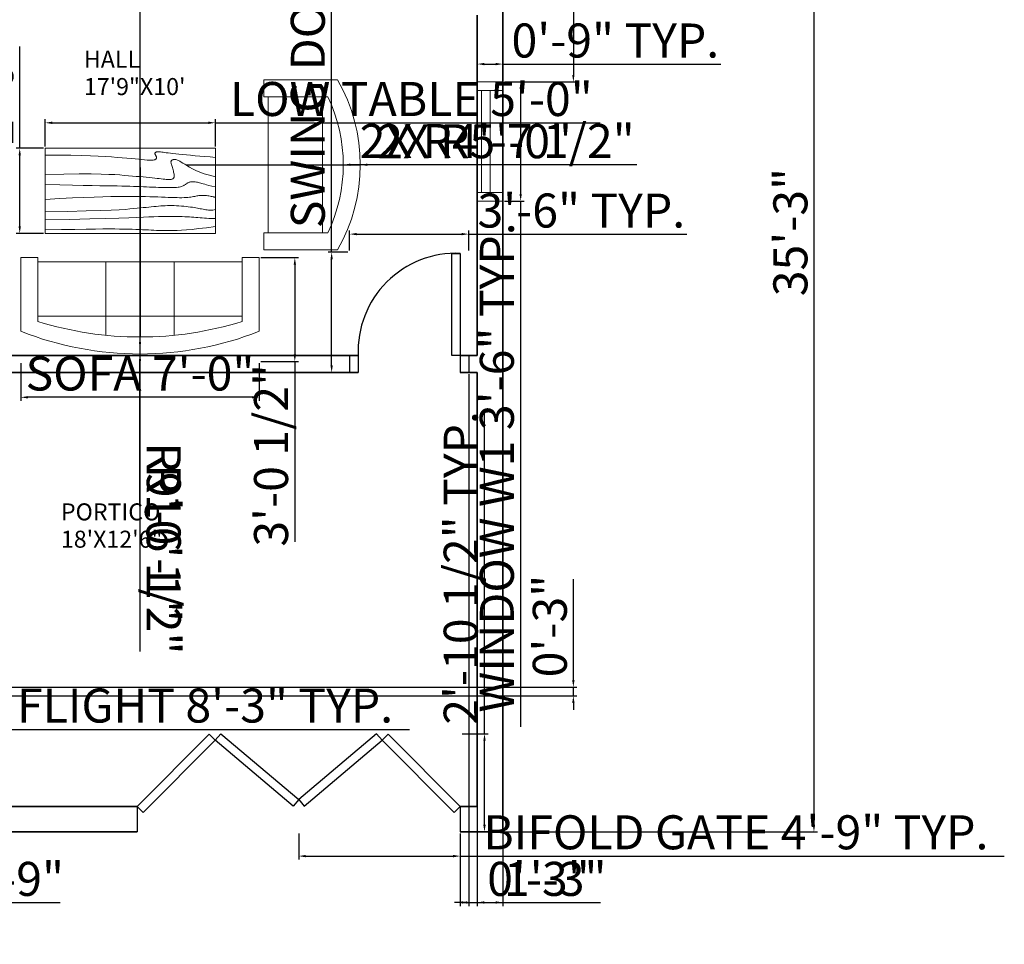
# Model space of a CAD drawing. Units: inches. Extents: x 2330 to 2931, y 514 to 1098.
# Tile 3 of 4: x 2583 to 2931, y 559 to 885. Entities that reach past the tile are written whole.
import ezdxf

# ---------------------------------------------------------------- set-up
doc = ezdxf.new("R2010")
doc.units = ezdxf.units.IN
for name, color, linetype, lineweight in [('A-ANNO-DIMS', 2, 'Continuous', 18), ('A-AREA-IDEN', 7, 'Continuous', 18), ('A-DOOR', 3, 'Continuous', 25), ('A-FURN', 8, 'Continuous', 18), ('A-GLAZ', 4, 'Continuous', 18), ('A-WALL', 7, 'Continuous', 35)]:
    doc.layers.add(name, color=color, linetype=linetype, lineweight=lineweight)
doc.styles.get("Standard").update_dxf_attribs({"font": 'arial.ttf'})
doc.dimstyles.new('ISO-25', dxfattribs={"dimtxt": 12, "dimasz": 2.5, "dimexe": 1.25, "dimexo": 0.625, "dimtad": 1, "dimdec": 1, "dimlunit": 3, "dimtxsty": 'Standard', "dimcen": 2.5, "dimadec": 0, "dimazin": 0, "dimtfac": 1, "dimtdec": 1, "dimtmove": 0, "dimatfit": 3, "dimfxl": 1, "dimarcsym": 0})

# ---------------------------------------------------------------- blocks, each defined once
blk = doc.blocks.new('*D2')
at = {"layer": 'A-ANNO-DIMS', "color": 0, "lineweight": -2, "transparency": 16777216}
for p, q in [((2754.43, 1021.47), (2864.79, 1021.47)), ((2863.54, 1018.97), (2863.54, 600.97)), ((2754.43, 598.47), (2864.79, 598.47))]:
    blk.add_line(p, q, dxfattribs=at)
at = {"layer": 'A-ANNO-DIMS', "color": 0, "transparency": 16777216}
for points in [[(2863.12, 1018.97), (2863.96, 1018.97), (2863.54, 1021.47)], [(2863.12, 600.97), (2863.96, 600.97), (2863.54, 598.47)]]:
    blk.add_solid(points, dxfattribs=at)
at = {"layer": 'Defpoints', "color": 0, "transparency": 16777216}
for p in [(2753.8, 1021.47), (2753.8, 598.47), (2863.54, 598.47)]:
    blk.add_point(p, dxfattribs=at)
at = {"layer": 'A-ANNO-DIMS', "color": 0, "transparency": 16777216, "insert": (2856.78, 809.97), "char_height": 12, "attachment_point": 5, "rotation": 90}
blk.add_mtext('35\'-3"', dxfattribs=at)
blk = doc.blocks.new('Table - Rectangular Woodgrain 60 x 30 in.')
for p, q in [((0, 0), (0, -30)), ((60, 0), (0, 0)), ((60, -30), (60, 0)), ((0, -30), (60, -30))]:
    blk.add_line(p, q)
for points in [[(0, -2.4), (4.8155, -2.418), (9.0302, -2.4688), (12.709, -2.5477), (15.9167, -2.65), (18.7181, -2.7711), (21.1781, -2.9063), (23.3616, -3.0508), (25.3333, -3.2), (27.1477, -3.3495), (28.8172, -3.4958), (30.3437, -3.636), (31.7291, -3.7667), (32.9756, -3.8849), (34.0849, -3.9875), (35.059, -4.0714), (35.9, -4.1334), (36.6114, -4.1711), (37.2041, -4.1854), (37.6906, -4.1779), (38.0833, -4.15), (38.3948, -4.1034), (38.6375, -4.0396), (38.8239, -3.9602), (38.9666, -3.8667), (39.0764, -3.7608), (39.1573, -3.6448), (39.2116, -3.521), (39.2416, -3.3917), (39.2498, -3.2593), (39.2385, -3.1261), (39.21, -2.9944), (39.1666, -2.8667), (39.111, -2.7447), (39.0468, -2.6281), (38.978, -2.5163), (38.9083, -2.4083), (38.8418, -2.3035), (38.7823, -2.201), (38.7337, -2.1001), (38.7, -2), (38.6844, -1.9003), (38.6875, -1.8021), (38.7094, -1.707), (38.75, -1.6167), (38.8094, -1.5326), (38.8875, -1.4563), (38.9844, -1.3893), (39.1, -1.3333), (39.2351, -1.2896), (39.3937, -1.2583), (39.5804, -1.2396), (39.8, -1.2333), (40.057, -1.2396), (40.3562, -1.2583), (40.7023, -1.2896), (41.1, -1.3333), (41.5547, -1.3895), (42.0755, -1.4573), (42.6721, -1.5361), (43.3542, -1.625), (44.1316, -1.7233), (45.014, -1.8302), (46.0114, -1.9449), (47.1333, -2.0667), (48.3862, -2.1947), (49.7625, -2.3281), (51.2513, -2.4663), (52.8416, -2.6083), (54.5226, -2.7535), (56.2833, -2.9011), (58.1127, -3.0501), (60, -3.2)], [(0, -9.2), (6.5759, -9.0858), (11.9385, -9.0365), (16.2527, -9.0418), (19.6833, -9.0917), (22.3952, -9.1759), (24.5531, -9.2844), (26.322, -9.4069), (27.8666, -9.5333), (29.3241, -9.6553), (30.7203, -9.7719), (32.0532, -9.8837), (33.3208, -9.9917), (34.5213, -10.0965), (35.6526, -10.199), (36.7128, -10.2999), (37.7, -10.4), (38.6129, -10.4996), (39.4531, -10.5969), (40.223, -10.6895), (40.925, -10.775), (41.5613, -10.8512), (42.1344, -10.9156), (42.6465, -10.966), (43.1, -11), (43.4976, -11.0158), (43.8437, -11.0136), (44.143, -10.9942), (44.4, -10.9583), (44.6195, -10.9069), (44.8062, -10.8406), (44.9648, -10.7603), (45.1, -10.6667), (45.2155, -10.5598), (45.3114, -10.4365), (45.3871, -10.2929), (45.4416, -10.125), (45.4743, -9.929), (45.4844, -9.7011), (45.4709, -9.4371), (45.4333, -9.1333), (45.3716, -8.7883), (45.2896, -8.4104), (45.1919, -8.0107), (45.0833, -7.6), (44.9685, -7.1893), (44.8521, -6.7896), (44.7388, -6.4117), (44.6333, -6.0667), (44.54, -5.7628), (44.4614, -5.4979), (44.4001, -5.2675), (44.3583, -5.0667), (44.3384, -4.8909), (44.3427, -4.7354), (44.3736, -4.5956), (44.4333, -4.4667), (44.5236, -4.3453), (44.6427, -4.2333), (44.7884, -4.1339), (44.9583, -4.05), (45.1501, -3.9849), (45.3614, -3.9417), (45.59, -3.9234), (45.8333, -3.9333), (46.0915, -3.9749), (46.3734, -4.0531), (46.6906, -4.1736), (47.0542, -4.3417), (47.4756, -4.5629), (47.9661, -4.8427), (48.5372, -5.1866), (49.2, -5.6), (49.9676, -6.0844), (50.8594, -6.625), (51.8965, -7.2031), (53.1, -7.8), (54.491, -8.3969), (56.0906, -8.975), (57.9199, -9.5156), (60, -10)], [(0, -12.8), (5.1847, -12.9322), (9.6213, -13.0323), (13.3963, -13.1059), (16.5958, -13.1583), (19.3063, -13.1952), (21.614, -13.2219), (23.6054, -13.2439), (25.3666, -13.2667), (26.9728, -13.2947), (28.4531, -13.3281), (29.8256, -13.3663), (31.1083, -13.4083), (32.3191, -13.4535), (33.476, -13.501), (34.597, -13.5501), (35.7, -13.6), (36.7984, -13.6497), (37.8875, -13.6979), (38.9578, -13.743), (40, -13.7833), (41.0047, -13.8174), (41.9625, -13.8438), (42.864, -13.8607), (43.7, -13.8667), (44.4631, -13.8604), (45.1552, -13.8417), (45.7801, -13.8104), (46.3416, -13.7667), (46.8439, -13.7104), (47.2906, -13.6417), (47.6858, -13.5604), (48.0333, -13.4667), (48.3375, -13.3608), (48.6042, -13.2448), (48.8396, -13.121), (49.05, -12.9917), (49.2417, -12.8593), (49.4208, -12.7261), (49.5937, -12.5944), (49.7667, -12.4667), (49.9452, -12.3451), (50.1323, -12.2313), (50.3303, -12.1268), (50.5416, -12.0333), (50.7686, -11.9524), (51.0135, -11.8854), (51.2788, -11.8341), (51.5666, -11.8), (51.8785, -11.7843), (52.2116, -11.7865), (52.562, -11.8059), (52.926, -11.8417), (53.2998, -11.8931), (53.6795, -11.9594), (54.0614, -12.0397), (54.4416, -12.1333), (54.8223, -12.2401), (55.2293, -12.3625), (55.6942, -12.5037), (56.2489, -12.6667), (56.9251, -12.8547), (57.7545, -13.0708), (58.7689, -13.3182), (60, -13.6)], [(0, -18), (5.124, -17.7273), (9.6609, -17.5057), (13.6705, -17.3303), (17.2125, -17.1958), (20.3467, -17.0973), (23.1328, -17.0297), (25.6307, -16.9878), (27.9, -16.9667), (29.9928, -16.9617), (31.9302, -16.9703), (33.7254, -16.9907), (35.3917, -17.0208), (36.9423, -17.0588), (38.3906, -17.1026), (39.7499, -17.1503), (41.0333, -17.2), (42.2519, -17.2496), (43.4073, -17.2969), (44.4986, -17.3395), (45.525, -17.375), (46.4858, -17.4012), (47.3802, -17.4156), (48.2074, -17.416), (48.9667, -17.4), (49.6583, -17.3662), (50.2872, -17.3167), (50.8595, -17.2547), (51.3812, -17.1833), (51.8584, -17.1057), (52.2971, -17.025), (52.7034, -16.9443), (53.0833, -16.8667), (53.443, -16.7951), (53.789, -16.7313), (54.128, -16.6768), (54.4666, -16.6334), (54.8115, -16.6024), (55.1693, -16.5854), (55.5465, -16.5841), (55.95, -16.6), (56.3828, -16.6337), (56.8346, -16.6823), (57.2915, -16.7418), (57.7396, -16.8084), (58.165, -16.878), (58.5539, -16.9469), (58.8924, -17.0111), (59.1666, -17.0667), (59.3679, -17.1107), (59.5078, -17.1438), (59.6032, -17.1675), (59.6708, -17.1833), (59.7275, -17.193), (59.7901, -17.1979), (59.8753, -17.1998), (60, -17.2)], [(0, -22.4), (8.0098, -22.2501), (14.4094, -22.1011), (19.4168, -21.9535), (23.25, -21.8083), (26.1269, -21.6663), (28.2656, -21.5281), (29.884, -21.3947), (31.2, -21.2667), (32.3967, -21.1448), (33.5172, -21.0292), (34.5697, -20.9198), (35.5625, -20.8167), (36.5037, -20.7198), (37.4015, -20.6292), (38.2642, -20.5448), (39.1, -20.4667), (39.9164, -20.3951), (40.7187, -20.3313), (41.5117, -20.2768), (42.3, -20.2333), (43.0883, -20.2024), (43.8812, -20.1854), (44.6836, -20.1841), (45.5, -20.2), (46.3328, -20.234), (47.1747, -20.2844), (48.0163, -20.3488), (48.8479, -20.425), (49.66, -20.5106), (50.4429, -20.6031), (51.1872, -20.7004), (51.8833, -20.8), (52.5246, -20.8999), (53.1166, -20.9995), (53.6681, -21.0983), (54.1875, -21.1958), (54.6834, -21.2919), (55.1646, -21.3859), (55.6394, -21.4777), (56.1167, -21.5667), (56.6028, -21.6515), (57.0961, -21.7266), (57.5929, -21.7852), (58.0896, -21.8208), (58.5823, -21.8268), (59.0674, -21.7964), (59.5412, -21.723), (60, -21.6)], [(0, -25.2), (8.6355, -25.0504), (15.7026, -24.9031), (21.4049, -24.7606), (25.9458, -24.625), (29.529, -24.4988), (32.3578, -24.3844), (34.6359, -24.284), (36.5667, -24.2), (38.3213, -24.1341), (39.9417, -24.0854), (41.437, -24.0523), (42.8167, -24.0333), (44.0901, -24.0268), (45.2667, -24.0313), (46.3557, -24.0451), (47.3667, -24.0667), (48.309, -24.0947), (49.1928, -24.1287), (50.0284, -24.168), (50.826, -24.2125), (51.5959, -24.2617), (52.3483, -24.3151), (53.0935, -24.3725), (53.8417, -24.4334), (54.6009, -24.497), (55.3699, -24.561), (56.1454, -24.6226), (56.9239, -24.6792), (57.7021, -24.7279), (58.4764, -24.7662), (59.2435, -24.7911), (60, -24.8)], [(0, -28.8), (5.6867, -28.6681), (10.45, -28.5698), (14.407, -28.5012), (17.675, -28.4584), (20.3711, -28.4374), (22.6125, -28.4344), (24.5164, -28.4455), (26.2, -28.4667), (27.762, -28.4947), (29.2276, -28.5281), (30.6033, -28.5663), (31.8958, -28.6084), (33.1118, -28.6535), (34.2578, -28.7011), (35.3405, -28.7501), (36.3666, -28.8), (37.3443, -28.8497), (38.288, -28.8974), (39.2137, -28.9412), (40.1375, -28.9792), (41.0753, -29.0093), (42.0432, -29.0297), (43.0572, -29.0384), (44.1333, -29.0333), (45.2936, -29.0114), (46.5843, -28.9641), (48.0579, -28.8816), (49.7666, -28.7542), (51.7629, -28.5721), (54.0989, -28.3255), (56.8272, -28.0048), (60, -27.6)]]:
    blk.add_lwpolyline(points)
blk = doc.blocks.new('Sofa - Roundback 7 ft.')
for p, q in [((-12.00002, -32.4421), (-12.00003, -6.5971)), ((11.99997, -32.4421), (11.99998, -6.5971)), ((-36.000027, -34), (-36.000027, -11.4696)), ((-35.999844, -13.3819), (35.9998, -13.3819)), ((35.99998, -34), (35.99998, -11.4696)), ((-36.000027, -32.4421), (35.99998, -32.4421))]:
    blk.add_line(p, q)
for points in [[(-36.000027, -34), (-42.000027, -34), (-42.000027, -8)], [(41.99998, -8), (41.99998, -34), (35.99998, -34)]]:
    blk.add_lwpolyline(points)
for centre, radius, start, end in [((0, -114.25), 114.25, 68.43141, 111.5686), ((-0.00001, -127.1968), 121.1968, 72.72033, 107.2797)]:
    blk.add_arc(centre, radius, start, end)
blk = doc.blocks.new('Sofa - Roundback Loveseat 5 ft.')
for p, q in [((0, -32.44198), (0, -5.99998)), ((-24, -33.99998), (-24, -11.46958)), ((-23.9998, -13.38178), (23.99986, -13.38178)), ((24.00004, -33.99998), (24.00004, -11.46958)), ((-24, -32.44198), (24.00004, -32.44198))]:
    blk.add_line(p, q)
for points in [[(-24, -33.99998), (-30, -33.99998), (-30, -7.99998)], [(30.00004, -7.99998), (30.00004, -33.99998), (24.00004, -33.99998)]]:
    blk.add_lwpolyline(points)
for centre, radius, start, end in [((0, -60.24998), 60.24998, 60.13715, 119.8628), ((0, -61.38438), 55.38444, 64.32083, 115.6792)]:
    blk.add_arc(centre, radius, start, end)
blk = doc.blocks.new('DOOR-SWING-36IN')
for p, q in [((0, 6), (0, 0)), ((3, 6), (3, 0)), ((39, 6), (39, 0)), ((42, 6), (42, 0))]:
    blk.add_line(p, q)
blk.add_lwpolyline([(39, 6), (36, 6), (36, 42), (39, 42)], close=True)
blk.add_arc((37.5, 7.5), 34.53, 87.5104, 182.4896)
blk = doc.blocks.new('WIN-36IN')
for p, q in [((0, 9), (0, 0)), ((39, 9), (3, 9)), ((3, 9), (3, 0)), ((39, 0), (39, 9)), ((42, 0), (42, 9)), ((3, 4.5), (39, 4.5)), ((3, 1.5), (39, 1.5)), ((3, 0), (39, 0))]:
    blk.add_line(p, q)
blk = doc.blocks.new('GATE-BIFOLD-PAIR-OF-PANELS')
blk.add_line((56.99, 9), (56.99, 0))
for points in [[(0, 11.36), (1.94, 9.07), (29.41, 32.33), (27.47, 34.62)], [(56.99, 9), (54.87, 6.88), (29.41, 32.33), (31.53, 34.46)]]:
    blk.add_lwpolyline(points, close=True)
blk = doc.blocks.new('*D15')
at = {"layer": 'A-ANNO-DIMS', "color": 0, "lineweight": -2, "transparency": 16777216}
for p, q in [((2693.44, 802.89), (2693.44, 1024.11)), ((2699.18, 802.89), (2692.19, 802.89)), ((2693.44, 762.97), (2693.44, 800.39)), ((2699.18, 760.47), (2692.19, 760.47))]:
    blk.add_line(p, q, dxfattribs=at)
at = {"layer": 'A-ANNO-DIMS', "color": 0, "transparency": 16777216}
for points in [[(2693.02, 800.39), (2693.86, 800.39), (2693.44, 802.89)], [(2693.02, 762.97), (2693.86, 762.97), (2693.44, 760.47)]]:
    blk.add_solid(points, dxfattribs=at)
at = {"layer": 'Defpoints', "color": 0, "transparency": 16777216}
for p in [(2693.44, 802.89), (2699.8, 802.89), (2699.8, 760.47)]:
    blk.add_point(p, dxfattribs=at)
at = {"layer": 'A-ANNO-DIMS', "color": 0, "transparency": 16777216, "insert": (2686.6, 914.75), "char_height": 12, "attachment_point": 5, "rotation": 90}
blk.add_mtext('SWING DOOR 3\'-6 1/2" TYP.', dxfattribs=at)
blk = doc.blocks.new('*D16')
at = {"layer": 'A-ANNO-DIMS', "color": 0, "lineweight": -2, "transparency": 16777216}
for p, q in [((2699.8, 803.52), (2699.8, 810.51)), ((2702.3, 809.26), (2739.3, 809.26)), ((2741.8, 803.52), (2741.8, 810.51)), ((2741.8, 809.26), (2818.69, 809.26))]:
    blk.add_line(p, q, dxfattribs=at)
at = {"layer": 'A-ANNO-DIMS', "color": 0, "transparency": 16777216}
for points in [[(2702.3, 809.67), (2702.3, 808.84), (2699.8, 809.26)], [(2739.3, 809.67), (2739.3, 808.84), (2741.8, 809.26)]]:
    blk.add_solid(points, dxfattribs=at)
at = {"layer": 'Defpoints', "color": 0, "transparency": 16777216}
for p in [(2741.8, 809.26), (2699.8, 802.89), (2741.8, 802.89)]:
    blk.add_point(p, dxfattribs=at)
at = {"layer": 'A-ANNO-DIMS', "color": 0, "transparency": 16777216, "insert": (2781.5, 816.01), "char_height": 12, "attachment_point": 5}
blk.add_mtext('3\'-6" TYP.', dxfattribs=at)
blk = doc.blocks.new('*D17')
at = {"layer": 'A-ANNO-DIMS', "color": 0, "lineweight": -2, "transparency": 16777216}
for p, q in [((2754.43, 862.92), (2761.35, 862.92)), ((2760.1, 860.42), (2760.1, 823.42)), ((2754.43, 820.92), (2761.35, 820.92)), ((2760.1, 820.92), (2760.1, 635.52))]:
    blk.add_line(p, q, dxfattribs=at)
at = {"layer": 'A-ANNO-DIMS', "color": 0, "transparency": 16777216}
for points in [[(2759.69, 860.42), (2760.52, 860.42), (2760.1, 862.92)], [(2759.69, 823.42), (2760.52, 823.42), (2760.1, 820.92)]]:
    blk.add_solid(points, dxfattribs=at)
at = {"layer": 'Defpoints', "color": 0, "transparency": 16777216}
for p in [(2753.8, 862.92), (2753.8, 820.92), (2760.1, 820.92)]:
    blk.add_point(p, dxfattribs=at)
at = {"layer": 'A-ANNO-DIMS', "color": 0, "transparency": 16777216, "insert": (2753.26, 726.97), "char_height": 12, "attachment_point": 5, "rotation": 90}
blk.add_mtext('WINDOW W1 3\'-6" TYP.', dxfattribs=at)
blk = doc.blocks.new('*D18')
at = {"layer": 'A-ANNO-DIMS', "color": 0, "lineweight": -2, "transparency": 16777216}
for p, q in [((2744.8, 863.55), (2744.8, 870.47)), ((2747.3, 869.22), (2751.3, 869.22)), ((2753.8, 863.55), (2753.8, 870.47)), ((2753.8, 869.22), (2830.7, 869.22))]:
    blk.add_line(p, q, dxfattribs=at)
at = {"layer": 'A-ANNO-DIMS', "color": 0, "transparency": 16777216}
for points in [[(2747.3, 869.64), (2747.3, 868.8), (2744.8, 869.22)], [(2751.3, 869.64), (2751.3, 868.8), (2753.8, 869.22)]]:
    blk.add_solid(points, dxfattribs=at)
at = {"layer": 'Defpoints', "color": 0, "transparency": 16777216}
for p in [(2753.8, 869.22), (2744.8, 862.92), (2753.8, 862.92)]:
    blk.add_point(p, dxfattribs=at)
at = {"layer": 'A-ANNO-DIMS', "color": 0, "transparency": 16777216, "insert": (2793.5, 875.97), "char_height": 12, "attachment_point": 5}
blk.add_mtext('0\'-9" TYP.', dxfattribs=at)
blk = doc.blocks.new('*D27')
at = {"layer": 'A-ANNO-DIMS', "color": 0, "lineweight": -2, "transparency": 16777216}
for p, q in [((2681.82, 597.85), (2681.82, 588.67)), ((2738.8, 597.85), (2738.8, 588.67)), ((2684.32, 589.92), (2736.3, 589.92)), ((2738.8, 589.92), (2930.67, 589.92))]:
    blk.add_line(p, q, dxfattribs=at)
at = {"layer": 'A-ANNO-DIMS', "color": 0, "transparency": 16777216}
for points in [[(2684.32, 590.34), (2684.32, 589.51), (2681.82, 589.92)], [(2736.3, 590.34), (2736.3, 589.51), (2738.8, 589.92)]]:
    blk.add_solid(points, dxfattribs=at)
at = {"layer": 'Defpoints', "color": 0, "transparency": 16777216}
for p in [(2681.82, 598.47), (2738.8, 598.47), (2738.8, 589.92)]:
    blk.add_point(p, dxfattribs=at)
at = {"layer": 'A-ANNO-DIMS', "color": 0, "transparency": 16777216, "insert": (2835.99, 596.76), "char_height": 12, "attachment_point": 5}
blk.add_mtext('BIFOLD GATE 4\'-9" TYP.', dxfattribs=at)
blk = doc.blocks.new('*D28')
at = {"layer": 'A-ANNO-DIMS', "color": 0, "lineweight": -2, "transparency": 16777216}
for p, q in [((2747.35, 633.1), (2747.35, 747.48)), ((2739.43, 633.1), (2748.6, 633.1)), ((2747.35, 600.97), (2747.35, 630.6)), ((2739.43, 598.47), (2748.6, 598.47))]:
    blk.add_line(p, q, dxfattribs=at)
at = {"layer": 'A-ANNO-DIMS', "color": 0, "transparency": 16777216}
for points in [[(2746.93, 630.6), (2747.77, 630.6), (2747.35, 633.1)], [(2746.93, 600.97), (2747.77, 600.97), (2747.35, 598.47)]]:
    blk.add_solid(points, dxfattribs=at)
at = {"layer": 'Defpoints', "color": 0, "transparency": 16777216}
for p in [(2738.8, 633.1), (2747.35, 633.1), (2738.8, 598.47)]:
    blk.add_point(p, dxfattribs=at)
at = {"layer": 'A-ANNO-DIMS', "color": 0, "transparency": 16777216, "insert": (2740.52, 691.54), "char_height": 12, "attachment_point": 5, "rotation": 90}
blk.add_mtext('2\'-10 1/2" TYP.', dxfattribs=at)
blk = doc.blocks.new('*D29')
at = {"layer": 'A-ANNO-DIMS', "color": 0, "lineweight": -2, "transparency": 16777216}
for p, q in [((2426.8, 648.85), (2426.8, 633.37)), ((2525.8, 648.85), (2525.8, 633.37)), ((2429.3, 634.62), (2523.3, 634.62)), ((2525.8, 634.62), (2720.93, 634.62))]:
    blk.add_line(p, q, dxfattribs=at)
at = {"layer": 'A-ANNO-DIMS', "color": 0, "transparency": 16777216}
for points in [[(2429.3, 635.04), (2429.3, 634.21), (2426.8, 634.62)], [(2523.3, 635.04), (2523.3, 634.21), (2525.8, 634.62)]]:
    blk.add_solid(points, dxfattribs=at)
at = {"layer": 'Defpoints', "color": 0, "transparency": 16777216}
for p in [(2426.8, 649.47), (2525.8, 649.47), (2525.8, 634.62)]:
    blk.add_point(p, dxfattribs=at)
at = {"layer": 'A-ANNO-DIMS', "color": 0, "transparency": 16777216, "insert": (2624.62, 641.46), "char_height": 12, "attachment_point": 5}
blk.add_mtext('STAIR FLIGHT 8\'-3" TYP.', dxfattribs=at)
blk = doc.blocks.new('*D33')
at = {"layer": 'A-ANNO-DIMS', "color": 0, "lineweight": -2, "transparency": 16777216}
for p, q in [((2592.44, 840.13), (2592.44, 849.76)), ((2594.94, 848.51), (2649.94, 848.51)), ((2652.44, 840.13), (2652.44, 849.76)), ((2652.44, 848.51), (2788.17, 848.51))]:
    blk.add_line(p, q, dxfattribs=at)
at = {"layer": 'A-ANNO-DIMS', "color": 0, "transparency": 16777216}
for points in [[(2594.94, 848.93), (2594.94, 848.09), (2592.44, 848.51)], [(2649.94, 848.93), (2649.94, 848.09), (2652.44, 848.51)]]:
    blk.add_solid(points, dxfattribs=at)
at = {"layer": 'Defpoints', "color": 0, "transparency": 16777216}
for p in [(2652.44, 848.51), (2592.44, 839.51), (2652.44, 839.51)]:
    blk.add_point(p, dxfattribs=at)
at = {"layer": 'A-ANNO-DIMS', "color": 0, "transparency": 16777216, "insert": (2721.56, 855.34), "char_height": 12, "attachment_point": 5}
blk.add_mtext('LOW TABLE 5\'-0"', dxfattribs=at)
blk = doc.blocks.new('*D34')
at = {"layer": 'A-ANNO-DIMS', "color": 0, "lineweight": -2, "transparency": 16777216}
for p, q in [((2583.44, 839.51), (2583.44, 875.36)), ((2591.82, 839.51), (2582.19, 839.51)), ((2583.44, 812.01), (2583.44, 837.01)), ((2591.82, 809.51), (2582.19, 809.51))]:
    blk.add_line(p, q, dxfattribs=at)
at = {"layer": 'A-ANNO-DIMS', "color": 0, "transparency": 16777216}
for points in [[(2583.03, 837.01), (2583.86, 837.01), (2583.44, 839.51)], [(2583.03, 812.01), (2583.86, 812.01), (2583.44, 809.51)]]:
    blk.add_solid(points, dxfattribs=at)
at = {"layer": 'Defpoints', "color": 0, "transparency": 16777216}
for p in [(2583.44, 839.51), (2592.44, 839.51), (2592.44, 809.51)]:
    blk.add_point(p, dxfattribs=at)
at = {"layer": 'A-ANNO-DIMS', "color": 0, "transparency": 16777216, "insert": (2576.69, 858.69), "char_height": 12, "attachment_point": 5, "rotation": 90}
blk.add_mtext('2\'-6"', dxfattribs=at)
blk = doc.blocks.new('*D35')
at = {"layer": 'A-ANNO-DIMS', "color": 0, "lineweight": -2, "transparency": 16777216}
for p, q in [((2583.86, 763.69), (2583.86, 750.46)), ((2667.86, 763.69), (2667.86, 750.46)), ((2665.36, 751.71), (2586.36, 751.71))]:
    blk.add_line(p, q, dxfattribs=at)
at = {"layer": 'A-ANNO-DIMS', "color": 0, "transparency": 16777216}
for points in [[(2586.36, 752.13), (2586.36, 751.3), (2583.86, 751.71)], [(2665.36, 752.13), (2665.36, 751.3), (2667.86, 751.71)]]:
    blk.add_solid(points, dxfattribs=at)
at = {"layer": 'Defpoints', "color": 0, "transparency": 16777216}
for p in [(2583.86, 764.31), (2667.86, 764.31), (2583.86, 751.71)]:
    blk.add_point(p, dxfattribs=at)
at = {"layer": 'A-ANNO-DIMS', "color": 0, "transparency": 16777216, "insert": (2625.86, 758.55), "char_height": 12, "attachment_point": 5}
blk.add_mtext('SOFA 7\'-0"', dxfattribs=at)
blk = doc.blocks.new('*D36')
at = {"layer": 'A-ANNO-DIMS', "color": 0, "lineweight": -2, "transparency": 16777216}
for p, q in [((2668.49, 800.98), (2681.71, 800.98)), ((2680.46, 798.48), (2680.46, 766.81)), ((2668.49, 764.31), (2681.71, 764.31)), ((2680.46, 764.31), (2680.46, 700.71))]:
    blk.add_line(p, q, dxfattribs=at)
at = {"layer": 'A-ANNO-DIMS', "color": 0, "transparency": 16777216}
for points in [[(2680.05, 798.48), (2680.88, 798.48), (2680.46, 800.98)], [(2680.05, 766.81), (2680.88, 766.81), (2680.46, 764.31)]]:
    blk.add_solid(points, dxfattribs=at)
at = {"layer": 'Defpoints', "color": 0, "transparency": 16777216}
for p in [(2667.86, 800.98), (2667.86, 764.31), (2680.46, 764.31)]:
    blk.add_point(p, dxfattribs=at)
at = {"layer": 'A-ANNO-DIMS', "color": 0, "transparency": 16777216, "insert": (2673.63, 731.26), "char_height": 12, "attachment_point": 5, "rotation": 90}
blk.add_mtext('3\'-0 1/2"', dxfattribs=at)
blk = doc.blocks.new('*D46')
at = {"layer": 'A-ANNO-DIMS', "color": 0, "lineweight": -2, "transparency": 16777216}
for p, q in [((2754.43, 1021.47), (2779.95, 1021.47)), ((2778.7, 1018.97), (2778.7, 865.42)), ((2754.43, 862.92), (2779.95, 862.92))]:
    blk.add_line(p, q, dxfattribs=at)
at = {"layer": 'A-ANNO-DIMS', "color": 0, "transparency": 16777216}
for points in [[(2778.28, 1018.97), (2779.11, 1018.97), (2778.7, 1021.47)], [(2778.28, 865.42), (2779.11, 865.42), (2778.7, 862.92)]]:
    blk.add_solid(points, dxfattribs=at)
at = {"layer": 'Defpoints', "color": 0, "transparency": 16777216}
for p in [(2753.8, 1021.47), (2753.8, 862.92), (2778.7, 862.92)]:
    blk.add_point(p, dxfattribs=at)
at = {"layer": 'A-ANNO-DIMS', "color": 0, "transparency": 16777216, "insert": (2771.86, 942.2), "char_height": 12, "attachment_point": 5, "rotation": 90}
blk.add_mtext('13\'-2 1/2"', dxfattribs=at)
blk = doc.blocks.new('*D47')
at = {"layer": 'A-ANNO-DIMS', "color": 0, "lineweight": -2, "transparency": 16777216}
for p, q in [((2738.8, 597.85), (2738.8, 572.33)), ((2753.8, 597.85), (2753.8, 572.33)), ((2741.3, 573.58), (2751.3, 573.58)), ((2753.8, 573.58), (2788.32, 573.58))]:
    blk.add_line(p, q, dxfattribs=at)
at = {"layer": 'A-ANNO-DIMS', "color": 0, "transparency": 16777216}
for points in [[(2741.3, 574), (2741.3, 573.16), (2738.8, 573.58)], [(2751.3, 574), (2751.3, 573.16), (2753.8, 573.58)]]:
    blk.add_solid(points, dxfattribs=at)
at = {"layer": 'Defpoints', "color": 0, "transparency": 16777216}
for p in [(2738.8, 598.47), (2753.8, 598.47), (2753.8, 573.58)]:
    blk.add_point(p, dxfattribs=at)
at = {"layer": 'A-ANNO-DIMS', "color": 0, "transparency": 16777216, "insert": (2772.31, 580.34), "char_height": 12, "attachment_point": 5}
blk.add_mtext('1\'-3"', dxfattribs=at)
blk = doc.blocks.new('*D51')
at = {"layer": 'A-ANNO-DIMS', "color": 0, "lineweight": -2, "transparency": 16777216}
for p, q in [((2741.8, 759.85), (2741.8, 572.33)), ((2744.8, 759.85), (2744.8, 572.33)), ((2739.3, 573.58), (2736.8, 573.58)), ((2741.8, 573.58), (2744.8, 573.58)), ((2747.3, 573.58), (2782.95, 573.58))]:
    blk.add_line(p, q, dxfattribs=at)
at = {"layer": 'A-ANNO-DIMS', "color": 0, "transparency": 16777216}
for points in [[(2739.3, 574), (2739.3, 573.16), (2741.8, 573.58)], [(2747.3, 574), (2747.3, 573.16), (2744.8, 573.58)]]:
    blk.add_solid(points, dxfattribs=at)
at = {"layer": 'Defpoints', "color": 0, "transparency": 16777216}
for p in [(2741.8, 760.47), (2744.8, 760.47), (2744.8, 573.58)]:
    blk.add_point(p, dxfattribs=at)
at = {"layer": 'A-ANNO-DIMS', "color": 0, "transparency": 16777216, "insert": (2766.38, 580.34), "char_height": 12, "attachment_point": 5}
blk.add_mtext('0\'-3"', dxfattribs=at)
blk = doc.blocks.new('*D52')
at = {"layer": 'A-ANNO-DIMS', "color": 0, "lineweight": -2, "transparency": 16777216}
for p, q in [((2778.7, 651.97), (2778.7, 687.62)), ((2526.43, 649.47), (2779.95, 649.47)), ((2778.7, 646.47), (2778.7, 649.47)), ((2526.43, 646.47), (2779.95, 646.47)), ((2778.7, 643.97), (2778.7, 641.47))]:
    blk.add_line(p, q, dxfattribs=at)
at = {"layer": 'A-ANNO-DIMS', "color": 0, "transparency": 16777216}
for points in [[(2778.28, 651.97), (2779.11, 651.97), (2778.7, 649.47)], [(2778.28, 643.97), (2779.11, 643.97), (2778.7, 646.47)]]:
    blk.add_solid(points, dxfattribs=at)
at = {"layer": 'Defpoints', "color": 0, "transparency": 16777216}
for p in [(2525.8, 649.47), (2778.7, 649.47), (2525.8, 646.47)]:
    blk.add_point(p, dxfattribs=at)
at = {"layer": 'A-ANNO-DIMS', "color": 0, "transparency": 16777216, "insert": (2771.94, 671.05), "char_height": 12, "attachment_point": 5, "rotation": 90}
blk.add_mtext('0\'-3"', dxfattribs=at)
blk = doc.blocks.new('*D56')
at = {"layer": 'A-ANNO-DIMS', "color": 0, "lineweight": -2, "transparency": 16777216}
for p, q in [((2528.8, 945.85), (2528.8, 572.33)), ((2561.8, 945.85), (2561.8, 572.33)), ((2531.3, 573.58), (2559.3, 573.58)), ((2561.8, 573.58), (2597.66, 573.58))]:
    blk.add_line(p, q, dxfattribs=at)
at = {"layer": 'A-ANNO-DIMS', "color": 0, "transparency": 16777216}
for points in [[(2531.3, 574), (2531.3, 573.16), (2528.8, 573.58)], [(2559.3, 574), (2559.3, 573.16), (2561.8, 573.58)]]:
    blk.add_solid(points, dxfattribs=at)
at = {"layer": 'Defpoints', "color": 0, "transparency": 16777216}
for p in [(2528.8, 946.47), (2561.8, 946.47), (2561.8, 573.58)]:
    blk.add_point(p, dxfattribs=at)
at = {"layer": 'A-ANNO-DIMS', "color": 0, "transparency": 16777216, "insert": (2580.98, 580.33), "char_height": 12, "attachment_point": 5}
blk.add_mtext('2\'-9"', dxfattribs=at)
blk = doc.blocks.new('*D59')
at = {"layer": 'A-ANNO-DIMS', "color": 0, "lineweight": -2, "transparency": 16777216}
for p, q in [((2625.86, 894.18), (2625.87, 772.98)), ((2625.87, 673.28), (2625.87, 770.48))]:
    blk.add_line(p, q, dxfattribs=at)
at = {"layer": 'A-ANNO-DIMS', "color": 0, "transparency": 16777216}
blk.add_solid([(2626.28, 770.48), (2625.45, 770.48), (2625.87, 772.98)], dxfattribs=at)
at = {"layer": 'Defpoints', "color": 0, "transparency": 16777216}
for p in [(2625.86, 894.18), (2625.87, 772.98)]:
    blk.add_point(p, dxfattribs=at)
at = {"layer": 'A-ANNO-DIMS', "color": 0, "transparency": 16777216, "insert": (2632.62, 700.26), "char_height": 12, "attachment_point": 5, "rotation": 270.0001}
blk.add_mtext('R10\'-1"', dxfattribs=at)
blk = doc.blocks.new('*D60')
at = {"layer": 'A-ANNO-DIMS', "color": 0, "lineweight": -2, "transparency": 16777216}
for p, q in [((2625.86, 881.23), (2625.86, 766.98)), ((2625.87, 662.13), (2625.86, 764.48))]:
    blk.add_line(p, q, dxfattribs=at)
at = {"layer": 'A-ANNO-DIMS', "color": 0, "transparency": 16777216}
blk.add_solid([(2626.28, 764.48), (2625.45, 764.48), (2625.86, 766.98)], dxfattribs=at)
at = {"layer": 'Defpoints', "color": 0, "transparency": 16777216}
for p in [(2625.86, 881.23), (2625.86, 766.98)]:
    blk.add_point(p, dxfattribs=at)
at = {"layer": 'A-ANNO-DIMS', "color": 0, "transparency": 16777216, "insert": (2632.69, 698.43), "char_height": 12, "attachment_point": 5, "rotation": 270.0001}
blk.add_mtext('R9\'-6 1/2"', dxfattribs=at)
blk = doc.blocks.new('*D61')
at = {"layer": 'A-ANNO-DIMS', "color": 0, "lineweight": -2, "transparency": 16777216}
for p, q in [((2643.3, 833.71), (2703.55, 833.71)), ((2779.17, 833.71), (2706.05, 833.71))]:
    blk.add_line(p, q, dxfattribs=at)
at = {"layer": 'A-ANNO-DIMS', "color": 0, "transparency": 16777216}
blk.add_solid([(2706.05, 834.12), (2706.05, 833.29), (2703.55, 833.71)], dxfattribs=at)
at = {"layer": 'Defpoints', "color": 0, "transparency": 16777216}
for p in [(2643.3, 833.71), (2703.55, 833.71)]:
    blk.add_point(p, dxfattribs=at)
at = {"layer": 'A-ANNO-DIMS', "color": 0, "transparency": 16777216, "insert": (2743.86, 840.46), "char_height": 12, "attachment_point": 5, "rotation": 359.9996}
blk.add_mtext('2X R5\'-0"', dxfattribs=at)
blk = doc.blocks.new('*D62')
at = {"layer": 'A-ANNO-DIMS', "color": 0, "lineweight": -2, "transparency": 16777216}
for p, q in [((2642.16, 833.71), (2697.55, 833.71)), ((2801.13, 833.71), (2700.05, 833.71))]:
    blk.add_line(p, q, dxfattribs=at)
at = {"layer": 'A-ANNO-DIMS', "color": 0, "transparency": 16777216}
blk.add_solid([(2700.05, 834.12), (2700.05, 833.29), (2697.55, 833.71)], dxfattribs=at)
at = {"layer": 'Defpoints', "color": 0, "transparency": 16777216}
for p in [(2642.16, 833.71), (2697.55, 833.71)]:
    blk.add_point(p, dxfattribs=at)
at = {"layer": 'A-ANNO-DIMS', "color": 0, "transparency": 16777216, "insert": (2751.84, 840.54), "char_height": 12, "attachment_point": 5, "rotation": 359.9996}
blk.add_mtext('2X R4\'-7 1/2"', dxfattribs=at)

msp = doc.modelspace()

# ---------------------------------------------------------------- linework, layer by layer
at = {"layer": 'A-DOOR'}
msp.add_line((2741.8, 607.47), (2741.8, 598.47), dxfattribs=at)
at = {"layer": 'A-WALL'}
for p, q in [((2744.8, 766.47), (2744.8, 886.47)), ((2702.8, 766.47), (2528.8, 766.47)), ((2744.8, 766.47), (2738.8, 766.47)), ((2702.8, 760.47), (2528.8, 760.47)), ((2744.8, 760.47), (2738.8, 760.47)), ((2744.8, 607.47), (2744.8, 760.47)), ((2390.8, 607.47), (2624.83, 607.47)), ((2738.8, 607.47), (2744.8, 607.47))]:
    msp.add_line(p, q, dxfattribs=at)
msp.add_lwpolyline([(2738.8, 598.47), (2753.8, 598.47), (2753.8, 1021.47), (2381.8, 1021.47), (2381.8, 598.47), (2624.83, 598.47)], dxfattribs=at)

# ---------------------------------------------------------------- block references
at = {"layer": 'A-DOOR'}
for name, p in [('DOOR-SWING-36IN', (2699.8, 760.47)), ('GATE-BIFOLD-PAIR-OF-PANELS', (2681.82, 598.47))]:
    msp.add_blockref(name, p, dxfattribs=at)
at = {"layer": 'A-DOOR', "extrusion": (0, 0, -1), "zscale": -1}
msp.add_blockref('GATE-BIFOLD-PAIR-OF-PANELS', (-2681.82, 598.47), dxfattribs=at)
at = {"layer": 'A-FURN'}
for name, p, rotation in [('Sofa - Roundback Loveseat 5 ft.', (2703.55, 833.71), 270), ('Sofa - Roundback 7 ft.', (2625.86, 766.98), 180)]:
    msp.add_blockref(name, p, dxfattribs=dict(at, rotation=rotation))
msp.add_blockref('Table - Rectangular Woodgrain 60 x 30 in.', (2592.44, 839.51), dxfattribs=at)
at = {"layer": 'A-GLAZ', "rotation": 270.0000000000021}
msp.add_blockref('WIN-36IN', (2744.8, 862.92), dxfattribs=at)

# ---------------------------------------------------------------- texts
at = {"layer": 'A-AREA-IDEN'}
for s, p in [('HALL', (2606.07, 867.92)), ('17\'9"X10\'', (2606.07, 858.28)), ('PORTICO', (2597.97, 708.31)), ('18\'X12\'6"', (2597.97, 698.67))]:
    msp.add_text(s, height=6, dxfattribs=at).set_placement(p)

# ---------------------------------------------------------------- dimensions: what is measured, and where the dimension line sits
at = {"layer": 'A-ANNO-DIMS'}
for base, p1, p2, angle, text, picture, middle in [((2693.44, 802.89), (2699.8, 760.47), (2699.8, 802.89), 90, 'SWING DOOR <> TYP.', '*D15', (2686.6, 914.75)), ((2753.8, 869.22), (2744.8, 862.92), (2753.8, 862.92), 0, '<> TYP.', '*D18', (2793.5, 875.97)), ((2760.1, 820.92), (2753.8, 862.92), (2753.8, 820.92), 270, 'WINDOW W1 <> TYP.', '*D17', (2753.26, 726.97)), ((2583.86, 751.71), (2667.86, 764.31), (2583.86, 764.31), 180, 'SOFA <>', '*D35', (2625.86, 758.55)), ((2747.35, 633.1), (2738.8, 598.47), (2738.8, 633.1), 90, '<> TYP.', '*D28', (2740.52, 691.54))]:
    dim = msp.add_linear_dim(base=base, p1=p1, p2=p2, angle=angle, text=text, dimstyle='ISO-25', override={"dimdec": 1, "dimlfac": 1, "dimrnd": 0, "dimzin": 1, "dimdsep": 46, "dimlunit": 4, "dimfrac": 2}, dxfattribs=at)
    dim.commit()
    dim.dimension.update_dxf_attribs({"geometry": picture, "text_midpoint": middle})
for base, p1, p2, angle, override, picture, middle in [((2863.54, 598.47), (2753.8, 1021.47), (2753.8, 598.47), 90, {"dimclrd": 0, "dimclre": 0, "dimclrt": 0}, '*D2', (2856.78, 809.97)), ((2778.6953, 862.9209), (2753.8028, 1021.4722), (2753.8028, 862.9209), 90, {"dimdec": 1, "dimlfac": 1, "dimrnd": 0, "dimzin": 1, "dimdsep": 46, "dimlunit": 4, "dimfrac": 2}, '*D46', (2771.8615, 942.1965)), ((2583.44, 839.51), (2592.44, 809.51), (2592.44, 839.51), 90, {"dimdec": 1, "dimlfac": 1, "dimrnd": 0, "dimzin": 1, "dimdsep": 46, "dimlunit": 4, "dimfrac": 2}, '*D34', (2576.69, 858.69)), ((2680.46, 764.31), (2667.86, 800.98), (2667.86, 764.31), 270, {"dimdec": 1, "dimlfac": 1, "dimrnd": 0, "dimzin": 1, "dimdsep": 46, "dimlunit": 4, "dimfrac": 2}, '*D36', (2673.63, 731.26)), ((2778.7, 649.47), (2525.8, 646.47), (2525.8, 649.47), 90, {"dimdec": 1, "dimlfac": 1, "dimrnd": 0, "dimzin": 1, "dimdsep": 46, "dimlunit": 4, "dimfrac": 2}, '*D52', (2771.94, 671.05))]:
    dim = msp.add_linear_dim(base=base, p1=p1, p2=p2, angle=angle, dimstyle='ISO-25', override=override, dxfattribs=at)
    dim.commit()
    dim.dimension.update_dxf_attribs({"geometry": picture, "text_midpoint": middle})
for base, p1, p2, picture, middle in [((2561.8, 573.58), (2528.8, 946.47), (2561.8, 946.47), '*D56', (2580.98, 580.33)), ((2744.8, 573.58), (2741.8, 760.47), (2744.8, 760.47), '*D51', (2766.38, 580.34)), ((2753.8, 573.58), (2738.8, 598.47), (2753.8, 598.47), '*D47', (2772.31, 580.34))]:
    dim = msp.add_linear_dim(base=base, p1=p1, p2=p2, dimstyle='ISO-25', override={"dimdec": 1, "dimlfac": 1, "dimrnd": 0, "dimzin": 1, "dimdsep": 46, "dimlunit": 4, "dimfrac": 2}, dxfattribs=at)
    dim.commit()
    dim.dimension.update_dxf_attribs({"geometry": picture, "text_midpoint": middle})
for center, mpoint, picture, middle in [((2625.86, 894.18), (2625.86, 772.98), '*D59', (2625.87, 700.26)), ((2625.864779, 881.229812), (2625.865, 766.979812), '*D60', (2625.8651326, 698.429812))]:
    dim = msp.add_radius_dim(center=center, mpoint=mpoint, dimstyle='ISO-25', override={"dimdec": 1, "dimlfac": 1, "dimrnd": 0, "dimzin": 1, "dimdsep": 46, "dimlunit": 4, "dimfrac": 2}, dxfattribs=at)
    dim.commit()
    dim.dimension.update_dxf_attribs({"geometry": picture, "text_midpoint": middle, "dimtype": 164})
for base, p1, p2, text, picture, middle in [((2652.44, 848.51), (2592.44, 839.51), (2652.44, 839.51), 'LOW TABLE <>', '*D33', (2721.56, 855.34)), ((2741.8, 809.26), (2699.8, 802.89), (2741.8, 802.89), '<> TYP.', '*D16', (2781.5, 816.01)), ((2525.8, 634.62), (2426.8, 649.47), (2525.8, 649.47), 'STAIR FLIGHT <> TYP.', '*D29', (2624.62, 641.46)), ((2738.8, 589.92), (2681.82, 598.47), (2738.8, 598.47), 'BIFOLD GATE <> TYP.', '*D27', (2835.99, 596.76))]:
    dim = msp.add_linear_dim(base=base, p1=p1, p2=p2, text=text, dimstyle='ISO-25', override={"dimdec": 1, "dimlfac": 1, "dimrnd": 0, "dimzin": 1, "dimdsep": 46, "dimlunit": 4, "dimfrac": 2}, dxfattribs=at)
    dim.commit()
    dim.dimension.update_dxf_attribs({"geometry": picture, "text_midpoint": middle})
for center, mpoint, picture, middle in [((2642.16, 833.71), (2697.55, 833.71), '*D62', (2751.84, 840.54)), ((2643.29783, 833.70839), (2703.54781, 833.708), '*D61', (2743.85908, 840.45961))]:
    dim = msp.add_radius_dim(center=center, mpoint=mpoint, text='2X <>', dimstyle='ISO-25', override={"dimdec": 1, "dimlfac": 1, "dimrnd": 0, "dimzin": 1, "dimdsep": 46, "dimlunit": 4, "dimfrac": 2}, dxfattribs=at)
    dim.commit()
    dim.dimension.update_dxf_attribs({"geometry": picture, "text_midpoint": middle})

doc.saveas('drawing.dxf')
